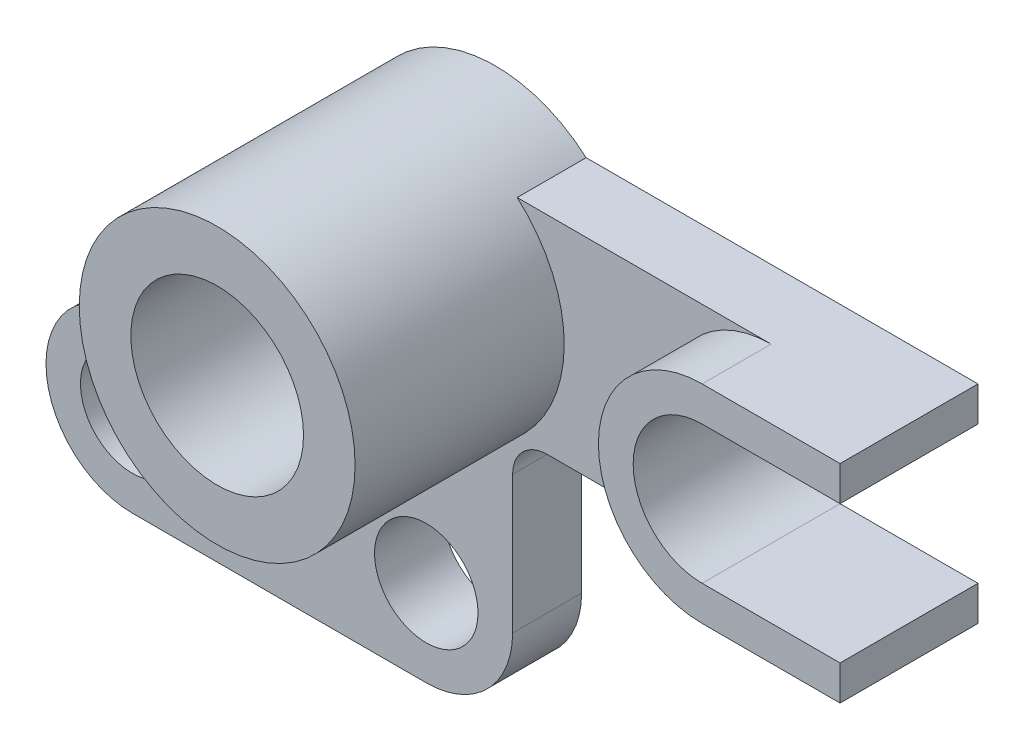
ISO-10303-21;
HEADER;
FILE_DESCRIPTION(('STEP AP214'),'2;1');
FILE_NAME('part.step','',(''),(''),'','','');
FILE_SCHEMA(('AUTOMOTIVE_DESIGN { 1 0 10303 214 1 1 1 1 }'));
ENDSEC;
DATA;
#1=APPLICATION_CONTEXT('core data for automotive mechanical design processes');
#2=APPLICATION_PROTOCOL_DEFINITION('international standard','automotive_design',2000,#1);
#3=PRODUCT_CONTEXT('',#1,'mechanical');
#4=PRODUCT('Part','Part','',(#3));
#5=PRODUCT_RELATED_PRODUCT_CATEGORY('part','',(#4));
#6=PRODUCT_DEFINITION_FORMATION('','',#4);
#7=PRODUCT_DEFINITION_CONTEXT('part definition',#1,'design');
#8=PRODUCT_DEFINITION('design','',#6,#7);
#9=PRODUCT_DEFINITION_SHAPE('','',#8);
#10=(LENGTH_UNIT() NAMED_UNIT(*) SI_UNIT(.MILLI.,.METRE.));
#11=(NAMED_UNIT(*) PLANE_ANGLE_UNIT() SI_UNIT($,.RADIAN.));
#12=(NAMED_UNIT(*) SI_UNIT($,.STERADIAN.) SOLID_ANGLE_UNIT());
#13=UNCERTAINTY_MEASURE_WITH_UNIT(LENGTH_MEASURE(1.E-05),#10,'distance_accuracy_value','');
#14=(GEOMETRIC_REPRESENTATION_CONTEXT(3) GLOBAL_UNCERTAINTY_ASSIGNED_CONTEXT((#13)) GLOBAL_UNIT_ASSIGNED_CONTEXT((#10,
#11,#12)) REPRESENTATION_CONTEXT('',''));
#15=CARTESIAN_POINT('',(0.,0.,0.));
#16=DIRECTION('',(0.,0.,1.));
#17=DIRECTION('',(1.,0.,0.));
#18=AXIS2_PLACEMENT_3D('',#15,#16,#17);
#19=CARTESIAN_POINT('',(0.,0.,25.6032));
#20=DIRECTION('',(0.,0.,-1.));
#21=DIRECTION('',(-1.,0.,0.));
#22=AXIS2_PLACEMENT_3D('',#19,#20,#21);
#23=CYLINDRICAL_SURFACE('',#22,12.7);
#24=CARTESIAN_POINT('',(0.,0.,25.6032));
#25=DIRECTION('',(0.,0.,1.));
#26=DIRECTION('',(1.,0.,0.));
#27=AXIS2_PLACEMENT_3D('',#24,#25,#26);
#28=CIRCLE('',#27,12.7);
#29=CARTESIAN_POINT('',(12.7,0.,25.6032));
#30=VERTEX_POINT('',#29);
#31=EDGE_CURVE('E11',#30,#30,#28,.T.);
#32=ORIENTED_EDGE('',*,*,#31,.F.);
#33=EDGE_LOOP('',(#32));
#34=FACE_BOUND('',#33,.T.);
#35=DIRECTION('',(0.,0.,-1.));
#36=VECTOR('',#35,1.);
#37=CARTESIAN_POINT('',(-12.7,0.,6.35));
#38=LINE('',#37,#36);
#39=CARTESIAN_POINT('',(-12.7,0.,6.35));
#40=VERTEX_POINT('',#39);
#41=CARTESIAN_POINT('',(-12.7,0.,0.));
#42=VERTEX_POINT('',#41);
#43=EDGE_CURVE('E52',#40,#42,#38,.T.);
#44=ORIENTED_EDGE('',*,*,#43,.F.);
#45=CARTESIAN_POINT('',(0.,0.,6.35));
#46=DIRECTION('',(0.,0.,-1.));
#47=DIRECTION('',(1.,0.,0.));
#48=AXIS2_PLACEMENT_3D('',#45,#46,#47);
#49=CIRCLE('',#48,12.7);
#50=CARTESIAN_POINT('',(8.37137144319854,9.5504,6.35));
#51=VERTEX_POINT('',#50);
#52=EDGE_CURVE('E204',#51,#40,#49,.T.);
#53=ORIENTED_EDGE('',*,*,#52,.F.);
#54=DIRECTION('',(0.,0.,-1.));
#55=VECTOR('',#54,1.);
#56=CARTESIAN_POINT('',(8.37137144319854,9.5504,6.35));
#57=LINE('',#56,#55);
#58=CARTESIAN_POINT('',(8.37137144319854,9.5504,0.));
#59=VERTEX_POINT('',#58);
#60=EDGE_CURVE('E227',#51,#59,#57,.T.);
#61=ORIENTED_EDGE('',*,*,#60,.T.);
#62=CARTESIAN_POINT('',(0.,0.,0.));
#63=DIRECTION('',(0.,0.,1.));
#64=DIRECTION('',(1.,0.,0.));
#65=AXIS2_PLACEMENT_3D('',#62,#63,#64);
#66=CIRCLE('',#65,12.7);
#67=EDGE_CURVE('E45',#59,#42,#66,.T.);
#68=ORIENTED_EDGE('',*,*,#67,.T.);
#69=EDGE_LOOP('',(#44,#53,#61,#68));
#70=FACE_BOUND('',#69,.T.);
#71=ADVANCED_FACE('F39',(#34,#70),#23,.T.);
#72=CARTESIAN_POINT('',(0.,0.,25.6032));
#73=DIRECTION('',(0.,0.,1.));
#74=DIRECTION('',(1.,0.,0.));
#75=AXIS2_PLACEMENT_3D('',#72,#73,#74);
#76=PLANE('',#75);
#77=ORIENTED_EDGE('',*,*,#31,.T.);
#78=EDGE_LOOP('',(#77));
#79=FACE_BOUND('',#78,.T.);
#80=CARTESIAN_POINT('',(0.,0.,25.6032));
#81=DIRECTION('',(0.,0.,1.));
#82=DIRECTION('',(1.,0.,0.));
#83=AXIS2_PLACEMENT_3D('',#80,#81,#82);
#84=CIRCLE('',#83,7.9502);
#85=CARTESIAN_POINT('',(7.9502,0.,25.6032));
#86=VERTEX_POINT('',#85);
#87=EDGE_CURVE('E280',#86,#86,#84,.T.);
#88=ORIENTED_EDGE('',*,*,#87,.F.);
#89=EDGE_LOOP('',(#88));
#90=FACE_BOUND('',#89,.T.);
#91=ADVANCED_FACE('F297',(#79,#90),#76,.T.);
#92=CARTESIAN_POINT('',(0.,0.,0.));
#93=DIRECTION('',(0.,0.,1.));
#94=DIRECTION('',(1.,0.,0.));
#95=AXIS2_PLACEMENT_3D('',#92,#93,#94);
#96=PLANE('',#95);
#97=ORIENTED_EDGE('',*,*,#67,.F.);
#98=DIRECTION('',(-1.,0.,0.));
#99=VECTOR('',#98,1.);
#100=CARTESIAN_POINT('',(31.75,9.55040000000001,0.));
#101=LINE('',#100,#99);
#102=CARTESIAN_POINT('',(44.45,9.5504,0.));
#103=VERTEX_POINT('',#102);
#104=EDGE_CURVE('E208',#103,#59,#101,.T.);
#105=ORIENTED_EDGE('',*,*,#104,.F.);
#106=DIRECTION('',(0.,1.,0.));
#107=VECTOR('',#106,1.);
#108=CARTESIAN_POINT('',(44.45,9.5504,0.));
#109=LINE('',#108,#107);
#110=CARTESIAN_POINT('',(44.45,6.35,0.));
#111=VERTEX_POINT('',#110);
#112=EDGE_CURVE('E182',#111,#103,#109,.T.);
#113=ORIENTED_EDGE('',*,*,#112,.F.);
#114=DIRECTION('',(1.,0.,0.));
#115=VECTOR('',#114,1.);
#116=CARTESIAN_POINT('',(44.45,6.35,0.));
#117=LINE('',#116,#115);
#118=CARTESIAN_POINT('',(31.75,6.35,0.));
#119=VERTEX_POINT('',#118);
#120=EDGE_CURVE('E524',#119,#111,#117,.T.);
#121=ORIENTED_EDGE('',*,*,#120,.F.);
#122=CARTESIAN_POINT('',(31.75,0.,0.));
#123=DIRECTION('',(0.,0.,-1.));
#124=DIRECTION('',(1.,0.,0.));
#125=AXIS2_PLACEMENT_3D('',#122,#123,#124);
#126=CIRCLE('',#125,6.35);
#127=CARTESIAN_POINT('',(31.75,-6.35,0.));
#128=VERTEX_POINT('',#127);
#129=EDGE_CURVE('E523',#128,#119,#126,.T.);
#130=ORIENTED_EDGE('',*,*,#129,.F.);
#131=DIRECTION('',(-1.,0.,0.));
#132=VECTOR('',#131,1.);
#133=CARTESIAN_POINT('',(31.75,-6.35,0.));
#134=LINE('',#133,#132);
#135=CARTESIAN_POINT('',(44.45,-6.35,0.));
#136=VERTEX_POINT('',#135);
#137=EDGE_CURVE('E519',#136,#128,#134,.T.);
#138=ORIENTED_EDGE('',*,*,#137,.F.);
#139=DIRECTION('',(0.,1.,0.));
#140=VECTOR('',#139,1.);
#141=CARTESIAN_POINT('',(44.45,-6.35,0.));
#142=LINE('',#141,#140);
#143=CARTESIAN_POINT('',(44.45,-9.5504,0.));
#144=VERTEX_POINT('',#143);
#145=EDGE_CURVE('E521',#144,#136,#142,.T.);
#146=ORIENTED_EDGE('',*,*,#145,.F.);
#147=DIRECTION('',(1.,0.,0.));
#148=VECTOR('',#147,1.);
#149=CARTESIAN_POINT('',(11.1252,-9.5504,0.));
#150=LINE('',#149,#148);
#151=CARTESIAN_POINT('',(11.1252,-9.55040000000001,0.));
#152=VERTEX_POINT('',#151);
#153=EDGE_CURVE('E246',#152,#144,#150,.T.);
#154=ORIENTED_EDGE('',*,*,#153,.F.);
#155=CARTESIAN_POINT('',(11.1252,-12.7254,0.));
#156=DIRECTION('',(0.,0.,-1.));
#157=DIRECTION('',(-1.,0.,0.));
#158=AXIS2_PLACEMENT_3D('',#155,#156,#157);
#159=CIRCLE('',#158,3.175);
#160=CARTESIAN_POINT('',(7.9502,-12.7254,0.));
#161=VERTEX_POINT('',#160);
#162=EDGE_CURVE('E243',#161,#152,#159,.T.);
#163=ORIENTED_EDGE('',*,*,#162,.F.);
#164=DIRECTION('',(0.,1.,0.));
#165=VECTOR('',#164,1.);
#166=CARTESIAN_POINT('',(7.9502,-25.3873,0.));
#167=LINE('',#166,#165);
#168=CARTESIAN_POINT('',(7.9502,-25.3873,0.));
#169=VERTEX_POINT('',#168);
#170=EDGE_CURVE('E241',#169,#161,#167,.T.);
#171=ORIENTED_EDGE('',*,*,#170,.F.);
#172=CARTESIAN_POINT('',(0.,-25.3873,0.));
#173=DIRECTION('',(0.,0.,1.));
#174=DIRECTION('',(1.,0.,0.));
#175=AXIS2_PLACEMENT_3D('',#172,#173,#174);
#176=CIRCLE('',#175,7.9502);
#177=CARTESIAN_POINT('',(0.,-33.3375,0.));
#178=VERTEX_POINT('',#177);
#179=EDGE_CURVE('E238',#178,#169,#176,.T.);
#180=ORIENTED_EDGE('',*,*,#179,.F.);
#181=DIRECTION('',(1.,0.,0.));
#182=VECTOR('',#181,1.);
#183=CARTESIAN_POINT('',(-27.0764,-33.3375,0.));
#184=LINE('',#183,#182);
#185=CARTESIAN_POINT('',(-27.0764,-33.3375,0.));
#186=VERTEX_POINT('',#185);
#187=EDGE_CURVE('E236',#186,#178,#184,.T.);
#188=ORIENTED_EDGE('',*,*,#187,.F.);
#189=CARTESIAN_POINT('',(-27.0764,-25.4,0.));
#190=DIRECTION('',(0.,0.,1.));
#191=DIRECTION('',(1.,0.,0.));
#192=AXIS2_PLACEMENT_3D('',#189,#190,#191);
#193=CIRCLE('',#192,7.9375);
#194=CARTESIAN_POINT('',(-27.0764,-17.4625,0.));
#195=VERTEX_POINT('',#194);
#196=EDGE_CURVE('E237',#195,#186,#193,.T.);
#197=ORIENTED_EDGE('',*,*,#196,.F.);
#198=DIRECTION('',(-1.,0.,0.));
#199=VECTOR('',#198,1.);
#200=CARTESIAN_POINT('',(-15.875,-17.4625,0.));
#201=LINE('',#200,#199);
#202=CARTESIAN_POINT('',(-15.875,-17.4625,0.));
#203=VERTEX_POINT('',#202);
#204=EDGE_CURVE('E232',#203,#195,#201,.T.);
#205=ORIENTED_EDGE('',*,*,#204,.F.);
#206=CARTESIAN_POINT('',(-15.875,-14.2875,0.));
#207=DIRECTION('',(0.,0.,-1.));
#208=DIRECTION('',(-1.,0.,0.));
#209=AXIS2_PLACEMENT_3D('',#206,#207,#208);
#210=CIRCLE('',#209,3.175);
#211=CARTESIAN_POINT('',(-12.7,-14.2875,0.));
#212=VERTEX_POINT('',#211);
#213=EDGE_CURVE('E235',#212,#203,#210,.T.);
#214=ORIENTED_EDGE('',*,*,#213,.F.);
#215=DIRECTION('',(0.,-1.,0.));
#216=VECTOR('',#215,1.);
#217=CARTESIAN_POINT('',(-12.7,0.,0.));
#218=LINE('',#217,#216);
#219=EDGE_CURVE('E203',#42,#212,#218,.T.);
#220=ORIENTED_EDGE('',*,*,#219,.F.);
#221=EDGE_LOOP('',(#97,#105,#113,#121,#130,#138,#146,#154,#163,#171,#180,#188,#197,#205,#214,#220));
#222=FACE_BOUND('',#221,.T.);
#223=CARTESIAN_POINT('',(0.,0.,0.));
#224=DIRECTION('',(0.,0.,1.));
#225=DIRECTION('',(1.,0.,0.));
#226=AXIS2_PLACEMENT_3D('',#223,#224,#225);
#227=CIRCLE('',#226,7.9502);
#228=CARTESIAN_POINT('',(7.9502,0.,0.));
#229=VERTEX_POINT('',#228);
#230=EDGE_CURVE('E277',#229,#229,#227,.T.);
#231=ORIENTED_EDGE('',*,*,#230,.T.);
#232=EDGE_LOOP('',(#231));
#233=FACE_BOUND('',#232,.T.);
#234=CARTESIAN_POINT('',(-27.0764,-25.4,0.));
#235=DIRECTION('',(0.,0.,1.));
#236=DIRECTION('',(1.,0.,0.));
#237=AXIS2_PLACEMENT_3D('',#234,#235,#236);
#238=CIRCLE('',#237,4.76250000000001);
#239=CARTESIAN_POINT('',(-22.3139,-25.4,0.));
#240=VERTEX_POINT('',#239);
#241=EDGE_CURVE('E198',#240,#240,#238,.T.);
#242=ORIENTED_EDGE('',*,*,#241,.T.);
#243=EDGE_LOOP('',(#242));
#244=FACE_BOUND('',#243,.T.);
#245=CARTESIAN_POINT('',(0.,-25.3873,0.));
#246=DIRECTION('',(0.,0.,1.));
#247=DIRECTION('',(1.,0.,0.));
#248=AXIS2_PLACEMENT_3D('',#245,#246,#247);
#249=CIRCLE('',#248,4.7625);
#250=CARTESIAN_POINT('',(4.76250000000001,-25.3873,0.));
#251=VERTEX_POINT('',#250);
#252=EDGE_CURVE('E189',#251,#251,#249,.T.);
#253=ORIENTED_EDGE('',*,*,#252,.T.);
#254=EDGE_LOOP('',(#253));
#255=FACE_BOUND('',#254,.T.);
#256=ADVANCED_FACE('F285',(#222,#233,#244,#255),#96,.F.);
#257=CARTESIAN_POINT('',(0.,0.,25.6032));
#258=DIRECTION('',(0.,0.,-1.));
#259=DIRECTION('',(-1.,0.,0.));
#260=AXIS2_PLACEMENT_3D('',#257,#258,#259);
#261=CYLINDRICAL_SURFACE('',#260,7.9502);
#262=ORIENTED_EDGE('',*,*,#87,.T.);
#263=EDGE_LOOP('',(#262));
#264=FACE_BOUND('',#263,.T.);
#265=ORIENTED_EDGE('',*,*,#230,.F.);
#266=EDGE_LOOP('',(#265));
#267=FACE_BOUND('',#266,.T.);
#268=ADVANCED_FACE('F286',(#264,#267),#261,.F.);
#269=CARTESIAN_POINT('',(0.,0.,6.35));
#270=DIRECTION('',(0.,0.,1.));
#271=DIRECTION('',(1.,0.,0.));
#272=AXIS2_PLACEMENT_3D('',#269,#270,#271);
#273=PLANE('',#272);
#274=CARTESIAN_POINT('',(-27.0764,-25.4,6.35));
#275=DIRECTION('',(0.,0.,1.));
#276=DIRECTION('',(1.,0.,0.));
#277=AXIS2_PLACEMENT_3D('',#274,#275,#276);
#278=CIRCLE('',#277,4.76250000000001);
#279=CARTESIAN_POINT('',(-22.3139,-25.4,6.35));
#280=VERTEX_POINT('',#279);
#281=EDGE_CURVE('E196',#280,#280,#278,.T.);
#282=ORIENTED_EDGE('',*,*,#281,.F.);
#283=EDGE_LOOP('',(#282));
#284=FACE_BOUND('',#283,.T.);
#285=ORIENTED_EDGE('',*,*,#52,.T.);
#286=DIRECTION('',(0.,-1.,0.));
#287=VECTOR('',#286,1.);
#288=CARTESIAN_POINT('',(-12.7,0.,6.35));
#289=LINE('',#288,#287);
#290=CARTESIAN_POINT('',(-12.7,-14.2875,6.35));
#291=VERTEX_POINT('',#290);
#292=EDGE_CURVE('E210',#40,#291,#289,.T.);
#293=ORIENTED_EDGE('',*,*,#292,.T.);
#294=CARTESIAN_POINT('',(-15.875,-14.2875,6.35));
#295=DIRECTION('',(0.,0.,-1.));
#296=DIRECTION('',(-1.,0.,0.));
#297=AXIS2_PLACEMENT_3D('',#294,#295,#296);
#298=CIRCLE('',#297,3.175);
#299=CARTESIAN_POINT('',(-15.875,-17.4625,6.35));
#300=VERTEX_POINT('',#299);
#301=EDGE_CURVE('E209',#291,#300,#298,.T.);
#302=ORIENTED_EDGE('',*,*,#301,.T.);
#303=DIRECTION('',(-1.,0.,0.));
#304=VECTOR('',#303,1.);
#305=CARTESIAN_POINT('',(-15.875,-17.4625,6.35));
#306=LINE('',#305,#304);
#307=CARTESIAN_POINT('',(-27.0764,-17.4625,6.35));
#308=VERTEX_POINT('',#307);
#309=EDGE_CURVE('E215',#300,#308,#306,.T.);
#310=ORIENTED_EDGE('',*,*,#309,.T.);
#311=CARTESIAN_POINT('',(-27.0764,-25.4,6.35));
#312=DIRECTION('',(0.,0.,1.));
#313=DIRECTION('',(1.,0.,0.));
#314=AXIS2_PLACEMENT_3D('',#311,#312,#313);
#315=CIRCLE('',#314,7.9375);
#316=CARTESIAN_POINT('',(-27.0764,-33.3375,6.35));
#317=VERTEX_POINT('',#316);
#318=EDGE_CURVE('E212',#308,#317,#315,.T.);
#319=ORIENTED_EDGE('',*,*,#318,.T.);
#320=DIRECTION('',(1.,0.,0.));
#321=VECTOR('',#320,1.);
#322=CARTESIAN_POINT('',(-27.0764,-33.3375,6.35));
#323=LINE('',#322,#321);
#324=CARTESIAN_POINT('',(0.,-33.3375,6.35));
#325=VERTEX_POINT('',#324);
#326=EDGE_CURVE('E216',#317,#325,#323,.T.);
#327=ORIENTED_EDGE('',*,*,#326,.T.);
#328=CARTESIAN_POINT('',(0.,-25.3873,6.35));
#329=DIRECTION('',(0.,0.,1.));
#330=DIRECTION('',(1.,0.,0.));
#331=AXIS2_PLACEMENT_3D('',#328,#329,#330);
#332=CIRCLE('',#331,7.9502);
#333=CARTESIAN_POINT('',(7.9502,-25.3873,6.35));
#334=VERTEX_POINT('',#333);
#335=EDGE_CURVE('E217',#325,#334,#332,.T.);
#336=ORIENTED_EDGE('',*,*,#335,.T.);
#337=DIRECTION('',(0.,1.,0.));
#338=VECTOR('',#337,1.);
#339=CARTESIAN_POINT('',(7.9502,-25.3873,6.35));
#340=LINE('',#339,#338);
#341=CARTESIAN_POINT('',(7.9502,-12.7254,6.35));
#342=VERTEX_POINT('',#341);
#343=EDGE_CURVE('E219',#334,#342,#340,.T.);
#344=ORIENTED_EDGE('',*,*,#343,.T.);
#345=CARTESIAN_POINT('',(11.1252,-12.7254,6.35));
#346=DIRECTION('',(0.,0.,-1.));
#347=DIRECTION('',(-1.,0.,0.));
#348=AXIS2_PLACEMENT_3D('',#345,#346,#347);
#349=CIRCLE('',#348,3.175);
#350=CARTESIAN_POINT('',(11.1252,-9.55040000000001,6.35));
#351=VERTEX_POINT('',#350);
#352=EDGE_CURVE('E225',#342,#351,#349,.T.);
#353=ORIENTED_EDGE('',*,*,#352,.T.);
#354=DIRECTION('',(1.,0.,0.));
#355=VECTOR('',#354,1.);
#356=CARTESIAN_POINT('',(11.1252,-9.5504,6.35));
#357=LINE('',#356,#355);
#358=CARTESIAN_POINT('',(31.75,-9.5504,6.35));
#359=VERTEX_POINT('',#358);
#360=EDGE_CURVE('E221',#351,#359,#357,.T.);
#361=ORIENTED_EDGE('',*,*,#360,.T.);
#362=CARTESIAN_POINT('',(31.75,0.,6.35));
#363=DIRECTION('',(0.,0.,-1.));
#364=DIRECTION('',(1.,0.,0.));
#365=AXIS2_PLACEMENT_3D('',#362,#363,#364);
#366=CIRCLE('',#365,9.5504);
#367=CARTESIAN_POINT('',(31.75,9.55040000000001,6.35));
#368=VERTEX_POINT('',#367);
#369=EDGE_CURVE('E183',#359,#368,#366,.T.);
#370=ORIENTED_EDGE('',*,*,#369,.T.);
#371=DIRECTION('',(-1.,0.,0.));
#372=VECTOR('',#371,1.);
#373=CARTESIAN_POINT('',(31.75,9.55040000000001,6.35));
#374=LINE('',#373,#372);
#375=EDGE_CURVE('E226',#368,#51,#374,.T.);
#376=ORIENTED_EDGE('',*,*,#375,.T.);
#377=EDGE_LOOP('',(#285,#293,#302,#310,#319,#327,#336,#344,#353,#361,#370,#376));
#378=FACE_BOUND('',#377,.T.);
#379=CARTESIAN_POINT('',(0.,-25.3873,6.35));
#380=DIRECTION('',(0.,0.,1.));
#381=DIRECTION('',(1.,0.,0.));
#382=AXIS2_PLACEMENT_3D('',#379,#380,#381);
#383=CIRCLE('',#382,4.7625);
#384=CARTESIAN_POINT('',(4.76250000000001,-25.3873,6.35));
#385=VERTEX_POINT('',#384);
#386=EDGE_CURVE('E188',#385,#385,#383,.T.);
#387=ORIENTED_EDGE('',*,*,#386,.F.);
#388=EDGE_LOOP('',(#387));
#389=FACE_BOUND('',#388,.T.);
#390=ADVANCED_FACE('F288',(#284,#378,#389),#273,.T.);
#391=CARTESIAN_POINT('',(-12.7,0.,6.35));
#392=DIRECTION('',(1.,0.,0.));
#393=DIRECTION('',(0.,1.,0.));
#394=AXIS2_PLACEMENT_3D('',#391,#392,#393);
#395=PLANE('',#394);
#396=ORIENTED_EDGE('',*,*,#219,.T.);
#397=DIRECTION('',(0.,0.,-1.));
#398=VECTOR('',#397,1.);
#399=CARTESIAN_POINT('',(-12.7,-14.2875,6.35));
#400=LINE('',#399,#398);
#401=EDGE_CURVE('E275',#291,#212,#400,.T.);
#402=ORIENTED_EDGE('',*,*,#401,.F.);
#403=ORIENTED_EDGE('',*,*,#292,.F.);
#404=ORIENTED_EDGE('',*,*,#43,.T.);
#405=EDGE_LOOP('',(#396,#402,#403,#404));
#406=FACE_BOUND('',#405,.T.);
#407=ADVANCED_FACE('F299',(#406),#395,.F.);
#408=CARTESIAN_POINT('',(-15.875,-14.2875,6.35));
#409=DIRECTION('',(0.,0.,-1.));
#410=DIRECTION('',(-1.,0.,0.));
#411=AXIS2_PLACEMENT_3D('',#408,#409,#410);
#412=CYLINDRICAL_SURFACE('',#411,3.175);
#413=ORIENTED_EDGE('',*,*,#213,.T.);
#414=DIRECTION('',(0.,0.,-1.));
#415=VECTOR('',#414,1.);
#416=CARTESIAN_POINT('',(-15.875,-17.4625,6.35));
#417=LINE('',#416,#415);
#418=EDGE_CURVE('E267',#300,#203,#417,.T.);
#419=ORIENTED_EDGE('',*,*,#418,.F.);
#420=ORIENTED_EDGE('',*,*,#301,.F.);
#421=ORIENTED_EDGE('',*,*,#401,.T.);
#422=EDGE_LOOP('',(#413,#419,#420,#421));
#423=FACE_BOUND('',#422,.T.);
#424=ADVANCED_FACE('F470',(#423),#412,.F.);
#425=CARTESIAN_POINT('',(-15.875,-17.4625,6.35));
#426=DIRECTION('',(0.,-1.,0.));
#427=DIRECTION('',(1.,0.,0.));
#428=AXIS2_PLACEMENT_3D('',#425,#426,#427);
#429=PLANE('',#428);
#430=ORIENTED_EDGE('',*,*,#204,.T.);
#431=DIRECTION('',(0.,0.,-1.));
#432=VECTOR('',#431,1.);
#433=CARTESIAN_POINT('',(-27.0764,-17.4625,6.35));
#434=LINE('',#433,#432);
#435=EDGE_CURVE('E266',#308,#195,#434,.T.);
#436=ORIENTED_EDGE('',*,*,#435,.F.);
#437=ORIENTED_EDGE('',*,*,#309,.F.);
#438=ORIENTED_EDGE('',*,*,#418,.T.);
#439=EDGE_LOOP('',(#430,#436,#437,#438));
#440=FACE_BOUND('',#439,.T.);
#441=ADVANCED_FACE('F465',(#440),#429,.F.);
#442=CARTESIAN_POINT('',(-27.0764,-25.4,6.35));
#443=DIRECTION('',(0.,0.,-1.));
#444=DIRECTION('',(-1.,0.,0.));
#445=AXIS2_PLACEMENT_3D('',#442,#443,#444);
#446=CYLINDRICAL_SURFACE('',#445,7.9375);
#447=ORIENTED_EDGE('',*,*,#196,.T.);
#448=DIRECTION('',(0.,0.,-1.));
#449=VECTOR('',#448,1.);
#450=CARTESIAN_POINT('',(-27.0764,-33.3375,6.35));
#451=LINE('',#450,#449);
#452=EDGE_CURVE('E263',#317,#186,#451,.T.);
#453=ORIENTED_EDGE('',*,*,#452,.F.);
#454=ORIENTED_EDGE('',*,*,#318,.F.);
#455=ORIENTED_EDGE('',*,*,#435,.T.);
#456=EDGE_LOOP('',(#447,#453,#454,#455));
#457=FACE_BOUND('',#456,.T.);
#458=ADVANCED_FACE('F459',(#457),#446,.T.);
#459=CARTESIAN_POINT('',(-27.0764,-33.3375,6.35));
#460=DIRECTION('',(0.,1.,0.));
#461=DIRECTION('',(0.,0.,1.));
#462=AXIS2_PLACEMENT_3D('',#459,#460,#461);
#463=PLANE('',#462);
#464=ORIENTED_EDGE('',*,*,#187,.T.);
#465=DIRECTION('',(0.,0.,-1.));
#466=VECTOR('',#465,1.);
#467=CARTESIAN_POINT('',(0.,-33.3375,6.35));
#468=LINE('',#467,#466);
#469=EDGE_CURVE('E257',#325,#178,#468,.T.);
#470=ORIENTED_EDGE('',*,*,#469,.F.);
#471=ORIENTED_EDGE('',*,*,#326,.F.);
#472=ORIENTED_EDGE('',*,*,#452,.T.);
#473=EDGE_LOOP('',(#464,#470,#471,#472));
#474=FACE_BOUND('',#473,.T.);
#475=ADVANCED_FACE('F454',(#474),#463,.F.);
#476=CARTESIAN_POINT('',(0.,-25.3873,6.35));
#477=DIRECTION('',(0.,0.,-1.));
#478=DIRECTION('',(-1.,0.,0.));
#479=AXIS2_PLACEMENT_3D('',#476,#477,#478);
#480=CYLINDRICAL_SURFACE('',#479,7.9502);
#481=ORIENTED_EDGE('',*,*,#179,.T.);
#482=DIRECTION('',(0.,0.,-1.));
#483=VECTOR('',#482,1.);
#484=CARTESIAN_POINT('',(7.9502,-25.3873,6.35));
#485=LINE('',#484,#483);
#486=EDGE_CURVE('E260',#334,#169,#485,.T.);
#487=ORIENTED_EDGE('',*,*,#486,.F.);
#488=ORIENTED_EDGE('',*,*,#335,.F.);
#489=ORIENTED_EDGE('',*,*,#469,.T.);
#490=EDGE_LOOP('',(#481,#487,#488,#489));
#491=FACE_BOUND('',#490,.T.);
#492=ADVANCED_FACE('F451',(#491),#480,.T.);
#493=CARTESIAN_POINT('',(7.9502,-25.3873,6.35));
#494=DIRECTION('',(-1.,0.,0.));
#495=DIRECTION('',(0.,0.,1.));
#496=AXIS2_PLACEMENT_3D('',#493,#494,#495);
#497=PLANE('',#496);
#498=ORIENTED_EDGE('',*,*,#170,.T.);
#499=DIRECTION('',(0.,0.,-1.));
#500=VECTOR('',#499,1.);
#501=CARTESIAN_POINT('',(7.9502,-12.7254,6.35));
#502=LINE('',#501,#500);
#503=EDGE_CURVE('E255',#342,#161,#502,.T.);
#504=ORIENTED_EDGE('',*,*,#503,.F.);
#505=ORIENTED_EDGE('',*,*,#343,.F.);
#506=ORIENTED_EDGE('',*,*,#486,.T.);
#507=EDGE_LOOP('',(#498,#504,#505,#506));
#508=FACE_BOUND('',#507,.T.);
#509=ADVANCED_FACE('F446',(#508),#497,.F.);
#510=CARTESIAN_POINT('',(11.1252,-12.7254,6.35));
#511=DIRECTION('',(0.,0.,-1.));
#512=DIRECTION('',(-1.,0.,0.));
#513=AXIS2_PLACEMENT_3D('',#510,#511,#512);
#514=CYLINDRICAL_SURFACE('',#513,3.175);
#515=ORIENTED_EDGE('',*,*,#162,.T.);
#516=DIRECTION('',(0.,0.,-1.));
#517=VECTOR('',#516,1.);
#518=CARTESIAN_POINT('',(11.1252,-9.55040000000001,6.35));
#519=LINE('',#518,#517);
#520=EDGE_CURVE('E253',#351,#152,#519,.T.);
#521=ORIENTED_EDGE('',*,*,#520,.F.);
#522=ORIENTED_EDGE('',*,*,#352,.F.);
#523=ORIENTED_EDGE('',*,*,#503,.T.);
#524=EDGE_LOOP('',(#515,#521,#522,#523));
#525=FACE_BOUND('',#524,.T.);
#526=ADVANCED_FACE('F441',(#525),#514,.F.);
#527=CARTESIAN_POINT('',(11.1252,-9.5504,6.35));
#528=DIRECTION('',(0.,1.,0.));
#529=DIRECTION('',(0.,0.,1.));
#530=AXIS2_PLACEMENT_3D('',#527,#528,#529);
#531=PLANE('',#530);
#532=ORIENTED_EDGE('',*,*,#153,.T.);
#533=DIRECTION('',(0.,0.,-1.));
#534=VECTOR('',#533,1.);
#535=CARTESIAN_POINT('',(44.45,-9.5504,12.7));
#536=LINE('',#535,#534);
#537=CARTESIAN_POINT('',(44.45,-9.5504,12.7));
#538=VERTEX_POINT('',#537);
#539=EDGE_CURVE('E166',#538,#144,#536,.T.);
#540=ORIENTED_EDGE('',*,*,#539,.F.);
#541=DIRECTION('',(1.,0.,0.));
#542=VECTOR('',#541,1.);
#543=CARTESIAN_POINT('',(44.45,-9.5504,12.7));
#544=LINE('',#543,#542);
#545=CARTESIAN_POINT('',(31.75,-9.5504,12.7));
#546=VERTEX_POINT('',#545);
#547=EDGE_CURVE('E161',#546,#538,#544,.T.);
#548=ORIENTED_EDGE('',*,*,#547,.F.);
#549=DIRECTION('',(0.,0.,-1.));
#550=VECTOR('',#549,1.);
#551=CARTESIAN_POINT('',(31.75,-9.5504,12.7));
#552=LINE('',#551,#550);
#553=EDGE_CURVE('E167',#546,#359,#552,.T.);
#554=ORIENTED_EDGE('',*,*,#553,.T.);
#555=ORIENTED_EDGE('',*,*,#360,.F.);
#556=ORIENTED_EDGE('',*,*,#520,.T.);
#557=EDGE_LOOP('',(#532,#540,#548,#554,#555,#556));
#558=FACE_BOUND('',#557,.T.);
#559=ADVANCED_FACE('F162',(#558),#531,.F.);
#560=CARTESIAN_POINT('',(31.75,9.55040000000001,6.35));
#561=DIRECTION('',(0.,-1.,0.));
#562=DIRECTION('',(1.,0.,0.));
#563=AXIS2_PLACEMENT_3D('',#560,#561,#562);
#564=PLANE('',#563);
#565=ORIENTED_EDGE('',*,*,#104,.T.);
#566=ORIENTED_EDGE('',*,*,#60,.F.);
#567=ORIENTED_EDGE('',*,*,#375,.F.);
#568=DIRECTION('',(0.,0.,-1.));
#569=VECTOR('',#568,1.);
#570=CARTESIAN_POINT('',(31.75,9.55040000000001,12.7));
#571=LINE('',#570,#569);
#572=CARTESIAN_POINT('',(31.75,9.55040000000001,12.7));
#573=VERTEX_POINT('',#572);
#574=EDGE_CURVE('E496',#573,#368,#571,.T.);
#575=ORIENTED_EDGE('',*,*,#574,.F.);
#576=DIRECTION('',(-1.,0.,0.));
#577=VECTOR('',#576,1.);
#578=CARTESIAN_POINT('',(31.75,9.55040000000001,12.7));
#579=LINE('',#578,#577);
#580=CARTESIAN_POINT('',(44.45,9.5504,12.7));
#581=VERTEX_POINT('',#580);
#582=EDGE_CURVE('E178',#581,#573,#579,.T.);
#583=ORIENTED_EDGE('',*,*,#582,.F.);
#584=DIRECTION('',(0.,0.,-1.));
#585=VECTOR('',#584,1.);
#586=CARTESIAN_POINT('',(44.45,9.5504,12.7));
#587=LINE('',#586,#585);
#588=EDGE_CURVE('E497',#581,#103,#587,.T.);
#589=ORIENTED_EDGE('',*,*,#588,.T.);
#590=EDGE_LOOP('',(#565,#566,#567,#575,#583,#589));
#591=FACE_BOUND('',#590,.T.);
#592=ADVANCED_FACE('F400',(#591),#564,.F.);
#593=CARTESIAN_POINT('',(-27.0764,-25.4,6.35));
#594=DIRECTION('',(0.,0.,-1.));
#595=DIRECTION('',(-1.,0.,0.));
#596=AXIS2_PLACEMENT_3D('',#593,#594,#595);
#597=CYLINDRICAL_SURFACE('',#596,4.76250000000001);
#598=ORIENTED_EDGE('',*,*,#281,.T.);
#599=EDGE_LOOP('',(#598));
#600=FACE_BOUND('',#599,.T.);
#601=ORIENTED_EDGE('',*,*,#241,.F.);
#602=EDGE_LOOP('',(#601));
#603=FACE_BOUND('',#602,.T.);
#604=ADVANCED_FACE('F405',(#600,#603),#597,.F.);
#605=CARTESIAN_POINT('',(0.,-25.3873,6.35));
#606=DIRECTION('',(0.,0.,-1.));
#607=DIRECTION('',(-1.,0.,0.));
#608=AXIS2_PLACEMENT_3D('',#605,#606,#607);
#609=CYLINDRICAL_SURFACE('',#608,4.7625);
#610=ORIENTED_EDGE('',*,*,#386,.T.);
#611=EDGE_LOOP('',(#610));
#612=FACE_BOUND('',#611,.T.);
#613=ORIENTED_EDGE('',*,*,#252,.F.);
#614=EDGE_LOOP('',(#613));
#615=FACE_BOUND('',#614,.T.);
#616=ADVANCED_FACE('F343',(#612,#615),#609,.F.);
#617=CARTESIAN_POINT('',(31.75,0.,12.7));
#618=DIRECTION('',(0.,0.,-1.));
#619=DIRECTION('',(-1.,0.,0.));
#620=AXIS2_PLACEMENT_3D('',#617,#618,#619);
#621=CYLINDRICAL_SURFACE('',#620,9.5504);
#622=ORIENTED_EDGE('',*,*,#369,.F.);
#623=ORIENTED_EDGE('',*,*,#553,.F.);
#624=CARTESIAN_POINT('',(31.75,0.,12.7));
#625=DIRECTION('',(0.,0.,1.));
#626=DIRECTION('',(1.,0.,0.));
#627=AXIS2_PLACEMENT_3D('',#624,#625,#626);
#628=CIRCLE('',#627,9.5504);
#629=EDGE_CURVE('E175',#573,#546,#628,.T.);
#630=ORIENTED_EDGE('',*,*,#629,.F.);
#631=ORIENTED_EDGE('',*,*,#574,.T.);
#632=EDGE_LOOP('',(#622,#623,#630,#631));
#633=FACE_BOUND('',#632,.T.);
#634=ADVANCED_FACE('F181',(#633),#621,.T.);
#635=CARTESIAN_POINT('',(44.45,-6.35,12.7));
#636=DIRECTION('',(-1.,0.,0.));
#637=DIRECTION('',(0.,0.,1.));
#638=AXIS2_PLACEMENT_3D('',#635,#636,#637);
#639=PLANE('',#638);
#640=ORIENTED_EDGE('',*,*,#145,.T.);
#641=DIRECTION('',(0.,0.,-1.));
#642=VECTOR('',#641,1.);
#643=CARTESIAN_POINT('',(44.45,-6.35,12.7));
#644=LINE('',#643,#642);
#645=CARTESIAN_POINT('',(44.45,-6.35,12.7));
#646=VERTEX_POINT('',#645);
#647=EDGE_CURVE('E191',#646,#136,#644,.T.);
#648=ORIENTED_EDGE('',*,*,#647,.F.);
#649=DIRECTION('',(0.,1.,0.));
#650=VECTOR('',#649,1.);
#651=CARTESIAN_POINT('',(44.45,-6.35,12.7));
#652=LINE('',#651,#650);
#653=EDGE_CURVE('E171',#538,#646,#652,.T.);
#654=ORIENTED_EDGE('',*,*,#653,.F.);
#655=ORIENTED_EDGE('',*,*,#539,.T.);
#656=EDGE_LOOP('',(#640,#648,#654,#655));
#657=FACE_BOUND('',#656,.T.);
#658=ADVANCED_FACE('F345',(#657),#639,.F.);
#659=CARTESIAN_POINT('',(31.75,-6.35,12.7));
#660=DIRECTION('',(0.,-1.,0.));
#661=DIRECTION('',(0.,0.,-1.));
#662=AXIS2_PLACEMENT_3D('',#659,#660,#661);
#663=PLANE('',#662);
#664=ORIENTED_EDGE('',*,*,#137,.T.);
#665=DIRECTION('',(0.,0.,-1.));
#666=VECTOR('',#665,1.);
#667=CARTESIAN_POINT('',(31.75,-6.35,12.7));
#668=LINE('',#667,#666);
#669=CARTESIAN_POINT('',(31.75,-6.35,12.7));
#670=VERTEX_POINT('',#669);
#671=EDGE_CURVE('E507',#670,#128,#668,.T.);
#672=ORIENTED_EDGE('',*,*,#671,.F.);
#673=DIRECTION('',(-1.,0.,0.));
#674=VECTOR('',#673,1.);
#675=CARTESIAN_POINT('',(31.75,-6.35,12.7));
#676=LINE('',#675,#674);
#677=EDGE_CURVE('E516',#646,#670,#676,.T.);
#678=ORIENTED_EDGE('',*,*,#677,.F.);
#679=ORIENTED_EDGE('',*,*,#647,.T.);
#680=EDGE_LOOP('',(#664,#672,#678,#679));
#681=FACE_BOUND('',#680,.T.);
#682=ADVANCED_FACE('F354',(#681),#663,.F.);
#683=CARTESIAN_POINT('',(31.75,0.,12.7));
#684=DIRECTION('',(0.,0.,-1.));
#685=DIRECTION('',(-1.,0.,0.));
#686=AXIS2_PLACEMENT_3D('',#683,#684,#685);
#687=CYLINDRICAL_SURFACE('',#686,6.35);
#688=ORIENTED_EDGE('',*,*,#129,.T.);
#689=DIRECTION('',(0.,0.,-1.));
#690=VECTOR('',#689,1.);
#691=CARTESIAN_POINT('',(31.75,6.35,12.7));
#692=LINE('',#691,#690);
#693=CARTESIAN_POINT('',(31.75,6.35,12.7));
#694=VERTEX_POINT('',#693);
#695=EDGE_CURVE('E501',#694,#119,#692,.T.);
#696=ORIENTED_EDGE('',*,*,#695,.F.);
#697=CARTESIAN_POINT('',(31.75,0.,12.7));
#698=DIRECTION('',(0.,0.,-1.));
#699=DIRECTION('',(1.,0.,0.));
#700=AXIS2_PLACEMENT_3D('',#697,#698,#699);
#701=CIRCLE('',#700,6.35);
#702=EDGE_CURVE('E532',#670,#694,#701,.T.);
#703=ORIENTED_EDGE('',*,*,#702,.F.);
#704=ORIENTED_EDGE('',*,*,#671,.T.);
#705=EDGE_LOOP('',(#688,#696,#703,#704));
#706=FACE_BOUND('',#705,.T.);
#707=ADVANCED_FACE('F359',(#706),#687,.F.);
#708=CARTESIAN_POINT('',(44.45,6.35,12.7));
#709=DIRECTION('',(0.,1.,0.));
#710=DIRECTION('',(-1.,0.,0.));
#711=AXIS2_PLACEMENT_3D('',#708,#709,#710);
#712=PLANE('',#711);
#713=ORIENTED_EDGE('',*,*,#120,.T.);
#714=DIRECTION('',(0.,0.,-1.));
#715=VECTOR('',#714,1.);
#716=CARTESIAN_POINT('',(44.45,6.35,12.7));
#717=LINE('',#716,#715);
#718=CARTESIAN_POINT('',(44.45,6.35,12.7));
#719=VERTEX_POINT('',#718);
#720=EDGE_CURVE('E499',#719,#111,#717,.T.);
#721=ORIENTED_EDGE('',*,*,#720,.F.);
#722=DIRECTION('',(1.,0.,0.));
#723=VECTOR('',#722,1.);
#724=CARTESIAN_POINT('',(44.45,6.35,12.7));
#725=LINE('',#724,#723);
#726=EDGE_CURVE('E531',#694,#719,#725,.T.);
#727=ORIENTED_EDGE('',*,*,#726,.F.);
#728=ORIENTED_EDGE('',*,*,#695,.T.);
#729=EDGE_LOOP('',(#713,#721,#727,#728));
#730=FACE_BOUND('',#729,.T.);
#731=ADVANCED_FACE('F369',(#730),#712,.F.);
#732=CARTESIAN_POINT('',(44.45,9.5504,12.7));
#733=DIRECTION('',(-1.,0.,0.));
#734=DIRECTION('',(0.,0.,1.));
#735=AXIS2_PLACEMENT_3D('',#732,#733,#734);
#736=PLANE('',#735);
#737=ORIENTED_EDGE('',*,*,#112,.T.);
#738=ORIENTED_EDGE('',*,*,#588,.F.);
#739=DIRECTION('',(0.,1.,0.));
#740=VECTOR('',#739,1.);
#741=CARTESIAN_POINT('',(44.45,9.5504,12.7));
#742=LINE('',#741,#740);
#743=EDGE_CURVE('E540',#719,#581,#742,.T.);
#744=ORIENTED_EDGE('',*,*,#743,.F.);
#745=ORIENTED_EDGE('',*,*,#720,.T.);
#746=EDGE_LOOP('',(#737,#738,#744,#745));
#747=FACE_BOUND('',#746,.T.);
#748=ADVANCED_FACE('F378',(#747),#736,.F.);
#749=CARTESIAN_POINT('',(31.75,0.,12.7));
#750=DIRECTION('',(0.,0.,1.));
#751=DIRECTION('',(1.,0.,0.));
#752=AXIS2_PLACEMENT_3D('',#749,#750,#751);
#753=PLANE('',#752);
#754=ORIENTED_EDGE('',*,*,#629,.T.);
#755=ORIENTED_EDGE('',*,*,#547,.T.);
#756=ORIENTED_EDGE('',*,*,#653,.T.);
#757=ORIENTED_EDGE('',*,*,#677,.T.);
#758=ORIENTED_EDGE('',*,*,#702,.T.);
#759=ORIENTED_EDGE('',*,*,#726,.T.);
#760=ORIENTED_EDGE('',*,*,#743,.T.);
#761=ORIENTED_EDGE('',*,*,#582,.T.);
#762=EDGE_LOOP('',(#754,#755,#756,#757,#758,#759,#760,#761));
#763=FACE_BOUND('',#762,.T.);
#764=ADVANCED_FACE('F176',(#763),#753,.T.);
#765=CLOSED_SHELL('',(#71,#91,#256,#268,#390,#407,#424,#441,#458,#475,#492,#509,#526,#559,#592,
#604,#616,#634,#658,#682,#707,#731,#748,#764));
#766=MANIFOLD_SOLID_BREP('B2',#765);
#767=ADVANCED_BREP_SHAPE_REPRESENTATION('',(#18,#766),#14);
#768=SHAPE_DEFINITION_REPRESENTATION(#9,#767);
ENDSEC;
END-ISO-10303-21;
